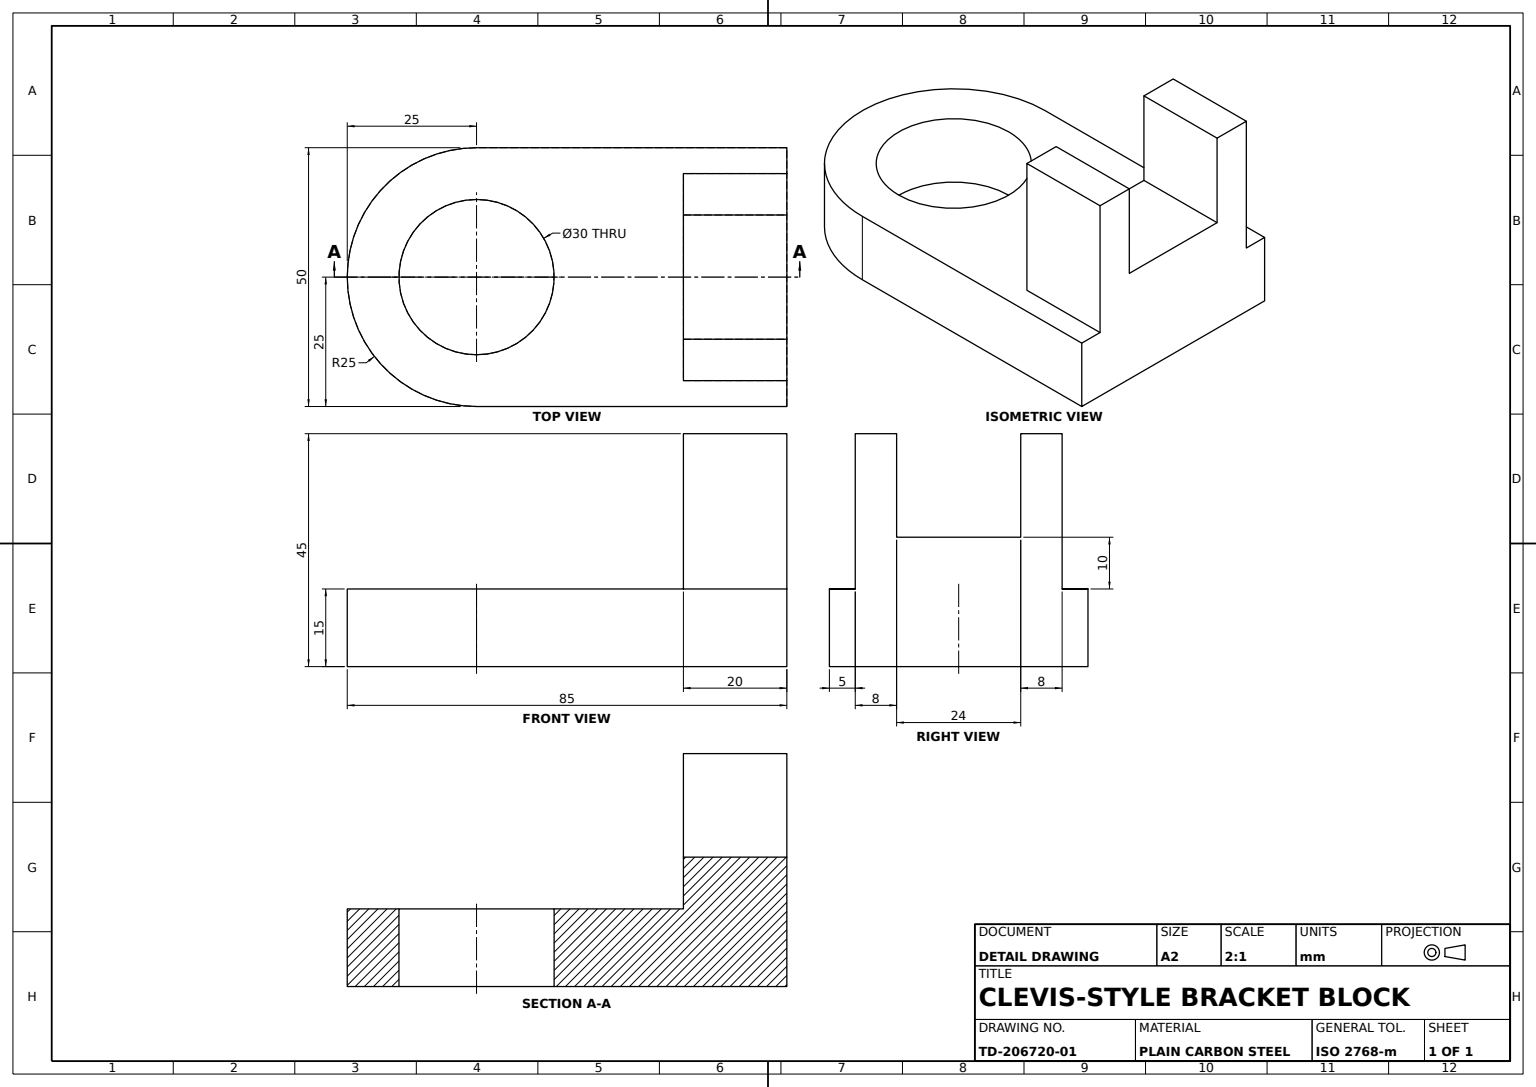
from build123d import *
from build123d.topology import SkipClean

# Parameters (mm, degrees)
BASE_BLOCK_SKETCH_W   = 60
BASE_BLOCK_SKETCH_H   = 15
BASE_BLOCK_DEPTH      = 25
FORK_UPRIGHT_DEPTH    = 20
ROUNDED_END_LUG_DEPTH = 15
BORE_SKETCH_R         = 15
BORE_30_DEPTH         = 15


with BuildPart() as part:
    # Base Block Sketch → Base Block (new, symmetric)
    with BuildSketch(Plane.XY):
        Rectangle(BASE_BLOCK_SKETCH_W, BASE_BLOCK_SKETCH_H)
    extrude(amount=BASE_BLOCK_DEPTH, both=True)

    # Fork Upright Sketch → Fork Upright (add)
    with BuildSketch(Plane(origin=(30, 0, 0), x_dir=(0, 0, -1), z_dir=(1, 0, 0))):
        Polygon((-20, 7.5), (-20, 37.5), (-12, 37.5), (-12, 17.5), (12, 17.5), (12, 37.5), (20, 37.5), (20, 7.5), align=None)
    extrude(amount=-FORK_UPRIGHT_DEPTH)

    # End Lug Sketch → Rounded End Lug (add)
    with BuildSketch(Plane(origin=(0, 7.5, 0), x_dir=(1, 0, 0), z_dir=(0, 1, 0))):
        with BuildLine():
            Line((-30, 15), (-30, 25))
            ThreePointArc((-30, 25), (-55, 0), (-30, -25))
            Line((-30, -25), (-30, -15))
            ThreePointArc((-30, -15), (-45, 0), (-30, 15))
        make_face()
    extrude(amount=-ROUNDED_END_LUG_DEPTH)

    # Bore Sketch → Bore Ø30 (cut)
    with SkipClean():  # the faces are left unmerged after this step: merging them gives an invalid solid
        with BuildSketch(Plane(origin=(0, 7.5, 0), x_dir=(1, 0, 0), z_dir=(0, 1, 0))):
            with Locations(Location((-30, 0, 0), (0, 0, 270))):
                Circle(BORE_SKETCH_R)
        extrude(amount=-BORE_30_DEPTH, mode=Mode.SUBTRACT)


solid = part.part
